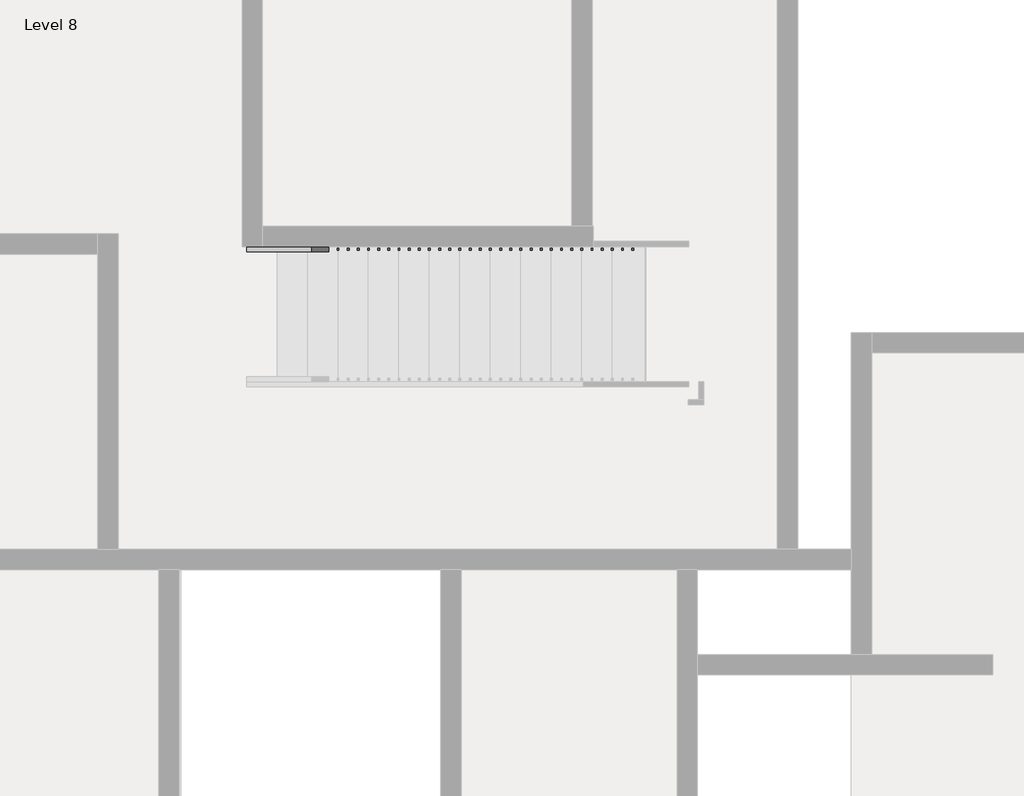
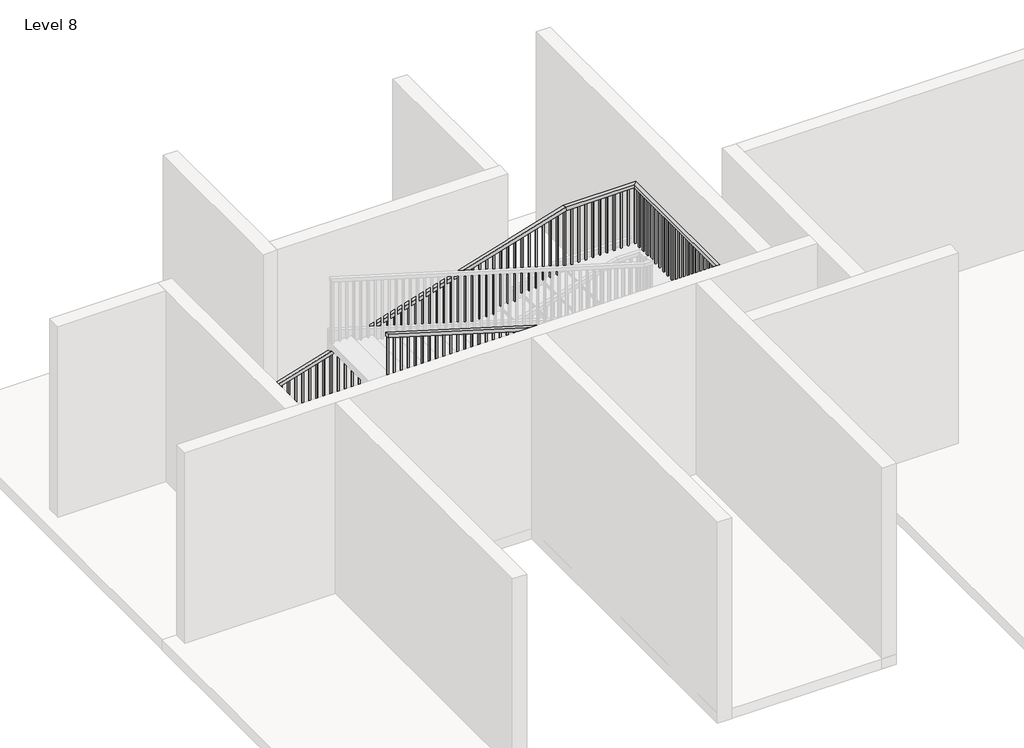
# One storey, part 10 of 14: 1 railing.
"""IFC4 building model written with IfcOpenShell, lengths in millimetres."""

from ifc_helpers import new_model, si_unit, frame, origin, place, context, project, spatial, polyline, outline, extrude, faceted_brep, element, save

model = new_model("IFC4")

# Units and contexts
model_context = context("Model", 3, world=origin())
ifc_project = project(units=[si_unit("LENGTHUNIT", "METRE", prefix="MILLI")], contexts=[model_context])

# Site, building, storey
site = spatial("IfcSite", under=ifc_project)
building = spatial("IfcBuilding", under=site)
storey = spatial("IfcBuildingStorey", under=building, Name="Level 8", Elevation=21336.0)

# Railing
placement = place(None, origin())
element("IfcRailing", 1, ObjectType="Handrail - Rectangular", at=placement, inside=storey, context=model_context, shape_type="SolidModel", body=[
    faceted_brep([(-5254.0891351, 12506.0715905, 22341.84), (-5254.0891351, 12506.0715905, 22288.8032429), (-5254.0891351, 12455.2715905, 22288.8032429), (-5254.0891351, 12455.2715905, 22341.84), (-986.8891351, 12506.0715905, 23622.0), (-979.4332782, 12506.0715905, 23571.2), (-979.4332782, 12455.2715905, 23571.2), (-986.8891351, 12455.2715905, 23622.0), (54.5108649, 12506.0715905, 23622.0), (54.5108649, 12506.0715905, 23571.2), (3.7108649, 12455.2715905, 23571.2), (3.7108649, 12455.2715905, 23622.0), (54.5108649, 9478.4949943, 23622.0), (54.5108649, 9478.4949943, 23571.2), (3.7108649, 9529.2949943, 23571.2), (3.7108649, 9529.2949943, 23622.0), (-682.0891351, 9478.4949943, 23622.0), (-689.544992, 9478.4949943, 23571.2), (-689.544992, 9529.2949943, 23571.2), (-682.0891351, 9529.2949943, 23622.0), (-5254.0891351, 9478.4949943, 24993.6), (-5254.0891351, 9529.2949943, 24993.6), (-5254.0891351, 9529.2949943, 24940.5632429), (-5254.0891351, 9478.4949943, 24940.5632429)], [[[0, 1, 2, 3]], [[1, 0, 4, 5]], [[2, 1, 5, 6]], [[3, 2, 6, 7]], [[0, 3, 7, 4]], [[5, 4, 8, 9]], [[6, 5, 9, 10]], [[7, 6, 10, 11]], [[4, 7, 11, 8]], [[9, 8, 12, 13]], [[10, 9, 13, 14]], [[11, 10, 14, 15]], [[8, 11, 15, 12]], [[13, 12, 16, 17]], [[14, 13, 17, 18]], [[15, 14, 18, 19]], [[12, 15, 19, 16]], [[20, 21, 22, 23]], [[17, 16, 20, 23]], [[18, 17, 23, 22]], [[19, 18, 22, 21]], [[16, 19, 21, 20]]]),
    extrude(outline(polyline([(24912.9407429, -5162.0141351), (23987.76, -5162.0141351), (23987.76, -5142.9641351), (24907.2257429, -5142.9641351), (24912.9407429, -5162.0141351)])), frame((0.0, 9494.3699943, 0.0), z_axis=(0.0, 1.0, 0.0), x_axis=(0.0, 0.0, 1.0)), (0.0, 0.0, 1.0), 19.05),
    extrude(outline(polyline([(24882.4607429, -5060.4141351), (23987.76, -5060.4141351), (23987.76, -5041.3641351), (24876.7457429, -5041.3641351), (24882.4607429, -5060.4141351)])), frame((0.0, 9494.3699943, 0.0), z_axis=(0.0, 1.0, 0.0), x_axis=(0.0, 0.0, 1.0)), (0.0, 0.0, 1.0), 19.05),
    extrude(outline(polyline([(24851.9807429, -4958.8141351), (23987.76, -4958.8141351), (23987.76, -4939.7641351), (24846.2657429, -4939.7641351), (24851.9807429, -4958.8141351)])), frame((0.0, 9494.3699943, 0.0), z_axis=(0.0, 1.0, 0.0), x_axis=(0.0, 0.0, 1.0)), (0.0, 0.0, 1.0), 19.05),
    extrude(outline(polyline([(24821.5007429, -4857.2141351), (23896.32, -4857.2141351), (23896.32, -4838.1641351), (24815.7857429, -4838.1641351), (24821.5007429, -4857.2141351)])), frame((0.0, 9494.3699943, 0.0), z_axis=(0.0, 1.0, 0.0), x_axis=(0.0, 0.0, 1.0)), (0.0, 0.0, 1.0), 19.05),
    extrude(outline(polyline([(24791.0207429, -4755.6141351), (23896.32, -4755.6141351), (23896.32, -4736.5641351), (24785.3057429, -4736.5641351), (24791.0207429, -4755.6141351)])), frame((0.0, 9494.3699943, 0.0), z_axis=(0.0, 1.0, 0.0), x_axis=(0.0, 0.0, 1.0)), (0.0, 0.0, 1.0), 19.05),
    extrude(outline(polyline([(24760.5407429, -4654.0141351), (23896.32, -4654.0141351), (23896.32, -4634.9641351), (24754.8257429, -4634.9641351), (24760.5407429, -4654.0141351)])), frame((0.0, 9494.3699943, 0.0), z_axis=(0.0, 1.0, 0.0), x_axis=(0.0, 0.0, 1.0)), (0.0, 0.0, 1.0), 19.05),
    extrude(outline(polyline([(24730.0607429, -4552.4141351), (23804.88, -4552.4141351), (23804.88, -4533.3641351), (24724.3457429, -4533.3641351), (24730.0607429, -4552.4141351)])), frame((0.0, 9494.3699943, 0.0), z_axis=(0.0, 1.0, 0.0), x_axis=(0.0, 0.0, 1.0)), (0.0, 0.0, 1.0), 19.05),
    extrude(outline(polyline([(24699.5807429, -4450.8141351), (23804.88, -4450.8141351), (23804.88, -4431.7641351), (24693.8657429, -4431.7641351), (24699.5807429, -4450.8141351)])), frame((0.0, 9494.3699943, 0.0), z_axis=(0.0, 1.0, 0.0), x_axis=(0.0, 0.0, 1.0)), (0.0, 0.0, 1.0), 19.05),
    extrude(outline(polyline([(24669.1007429, -4349.2141351), (23804.88, -4349.2141351), (23804.88, -4330.1641351), (24663.3857429, -4330.1641351), (24669.1007429, -4349.2141351)])), frame((0.0, 9494.3699943, 0.0), z_axis=(0.0, 1.0, 0.0), x_axis=(0.0, 0.0, 1.0)), (0.0, 0.0, 1.0), 19.05),
    extrude(outline(polyline([(24638.6207429, -4247.6141351), (23713.44, -4247.6141351), (23713.44, -4228.5641351), (24632.9057429, -4228.5641351), (24638.6207429, -4247.6141351)])), frame((0.0, 9494.3699943, 0.0), z_axis=(0.0, 1.0, 0.0), x_axis=(0.0, 0.0, 1.0)), (0.0, 0.0, 1.0), 19.05),
    extrude(outline(polyline([(24608.1407429, -4146.0141351), (23713.44, -4146.0141351), (23713.44, -4126.9641351), (24602.4257429, -4126.9641351), (24608.1407429, -4146.0141351)])), frame((0.0, 9494.3699943, 0.0), z_axis=(0.0, 1.0, 0.0), x_axis=(0.0, 0.0, 1.0)), (0.0, 0.0, 1.0), 19.05),
    extrude(outline(polyline([(24577.6607429, -4044.4141351), (23713.44, -4044.4141351), (23713.44, -4025.3641351), (24571.9457429, -4025.3641351), (24577.6607429, -4044.4141351)])), frame((0.0, 9494.3699943, 0.0), z_axis=(0.0, 1.0, 0.0), x_axis=(0.0, 0.0, 1.0)), (0.0, 0.0, 1.0), 19.05),
    extrude(outline(polyline([(24547.1807429, -3942.8141351), (23622.0, -3942.8141351), (23622.0, -3923.7641351), (24541.4657429, -3923.7641351), (24547.1807429, -3942.8141351)])), frame((0.0, 9494.3699943, 0.0), z_axis=(0.0, 1.0, 0.0), x_axis=(0.0, 0.0, 1.0)), (0.0, 0.0, 1.0), 19.05),
    extrude(outline(polyline([(24516.7007429, -3841.2141351), (23622.0, -3841.2141351), (23622.0, -3822.1641351), (24510.9857429, -3822.1641351), (24516.7007429, -3841.2141351)])), frame((0.0, 9494.3699943, 0.0), z_axis=(0.0, 1.0, 0.0), x_axis=(0.0, 0.0, 1.0)), (0.0, 0.0, 1.0), 19.05),
    extrude(outline(polyline([(24486.2207429, -3739.6141351), (23622.0, -3739.6141351), (23622.0, -3720.5641351), (24480.5057429, -3720.5641351), (24486.2207429, -3739.6141351)])), frame((0.0, 9494.3699943, 0.0), z_axis=(0.0, 1.0, 0.0), x_axis=(0.0, 0.0, 1.0)), (0.0, 0.0, 1.0), 19.05),
    extrude(outline(polyline([(24455.7407429, -3638.0141351), (23530.56, -3638.0141351), (23530.56, -3618.9641351), (24450.0257429, -3618.9641351), (24455.7407429, -3638.0141351)])), frame((0.0, 9494.3699943, 0.0), z_axis=(0.0, 1.0, 0.0), x_axis=(0.0, 0.0, 1.0)), (0.0, 0.0, 1.0), 19.05),
    extrude(outline(polyline([(24425.2607429, -3536.4141351), (23530.56, -3536.4141351), (23530.56, -3517.3641351), (24419.5457429, -3517.3641351), (24425.2607429, -3536.4141351)])), frame((0.0, 9494.3699943, 0.0), z_axis=(0.0, 1.0, 0.0), x_axis=(0.0, 0.0, 1.0)), (0.0, 0.0, 1.0), 19.05),
    extrude(outline(polyline([(24394.7807429, -3434.8141351), (23530.56, -3434.8141351), (23530.56, -3415.7641351), (24389.0657429, -3415.7641351), (24394.7807429, -3434.8141351)])), frame((0.0, 9494.3699943, 0.0), z_axis=(0.0, 1.0, 0.0), x_axis=(0.0, 0.0, 1.0)), (0.0, 0.0, 1.0), 19.05),
    extrude(outline(polyline([(24364.3007429, -3333.2141351), (23439.12, -3333.2141351), (23439.12, -3314.1641351), (24358.5857429, -3314.1641351), (24364.3007429, -3333.2141351)])), frame((0.0, 9494.3699943, 0.0), z_axis=(0.0, 1.0, 0.0), x_axis=(0.0, 0.0, 1.0)), (0.0, 0.0, 1.0), 19.05),
    extrude(outline(polyline([(24333.8207429, -3231.6141351), (23439.12, -3231.6141351), (23439.12, -3212.5641351), (24328.1057429, -3212.5641351), (24333.8207429, -3231.6141351)])), frame((0.0, 9494.3699943, 0.0), z_axis=(0.0, 1.0, 0.0), x_axis=(0.0, 0.0, 1.0)), (0.0, 0.0, 1.0), 19.05),
    extrude(outline(polyline([(24303.3407429, -3130.0141351), (23439.12, -3130.0141351), (23439.12, -3110.9641351), (24297.6257429, -3110.9641351), (24303.3407429, -3130.0141351)])), frame((0.0, 9494.3699943, 0.0), z_axis=(0.0, 1.0, 0.0), x_axis=(0.0, 0.0, 1.0)), (0.0, 0.0, 1.0), 19.05),
    extrude(outline(polyline([(24272.8607429, -3028.4141351), (23347.68, -3028.4141351), (23347.68, -3009.3641351), (24267.1457429, -3009.3641351), (24272.8607429, -3028.4141351)])), frame((0.0, 9494.3699943, 0.0), z_axis=(0.0, 1.0, 0.0), x_axis=(0.0, 0.0, 1.0)), (0.0, 0.0, 1.0), 19.05),
    extrude(outline(polyline([(24242.3807429, -2926.8141351), (23347.68, -2926.8141351), (23347.68, -2907.7641351), (24236.6657429, -2907.7641351), (24242.3807429, -2926.8141351)])), frame((0.0, 9494.3699943, 0.0), z_axis=(0.0, 1.0, 0.0), x_axis=(0.0, 0.0, 1.0)), (0.0, 0.0, 1.0), 19.05),
    extrude(outline(polyline([(24211.9007429, -2825.2141351), (23347.68, -2825.2141351), (23347.68, -2806.1641351), (24206.1857429, -2806.1641351), (24211.9007429, -2825.2141351)])), frame((0.0, 9494.3699943, 0.0), z_axis=(0.0, 1.0, 0.0), x_axis=(0.0, 0.0, 1.0)), (0.0, 0.0, 1.0), 19.05),
    extrude(outline(polyline([(24181.4207429, -2723.6141351), (23256.24, -2723.6141351), (23256.24, -2704.5641351), (24175.7057429, -2704.5641351), (24181.4207429, -2723.6141351)])), frame((0.0, 9494.3699943, 0.0), z_axis=(0.0, 1.0, 0.0), x_axis=(0.0, 0.0, 1.0)), (0.0, 0.0, 1.0), 19.05),
    extrude(outline(polyline([(24150.9407429, -2622.0141351), (23256.24, -2622.0141351), (23256.24, -2602.9641351), (24145.2257429, -2602.9641351), (24150.9407429, -2622.0141351)])), frame((0.0, 9494.3699943, 0.0), z_axis=(0.0, 1.0, 0.0), x_axis=(0.0, 0.0, 1.0)), (0.0, 0.0, 1.0), 19.05),
    extrude(outline(polyline([(24120.4607429, -2520.4141351), (23256.24, -2520.4141351), (23256.24, -2501.3641351), (24114.7457429, -2501.3641351), (24120.4607429, -2520.4141351)])), frame((0.0, 9494.3699943, 0.0), z_axis=(0.0, 1.0, 0.0), x_axis=(0.0, 0.0, 1.0)), (0.0, 0.0, 1.0), 19.05),
    extrude(outline(polyline([(24089.9807429, -2418.8141351), (23164.8, -2418.8141351), (23164.8, -2399.7641351), (24084.2657429, -2399.7641351), (24089.9807429, -2418.8141351)])), frame((0.0, 9494.3699943, 0.0), z_axis=(0.0, 1.0, 0.0), x_axis=(0.0, 0.0, 1.0)), (0.0, 0.0, 1.0), 19.05),
    extrude(outline(polyline([(24059.5007429, -2317.2141351), (23164.8, -2317.2141351), (23164.8, -2298.1641351), (24053.7857429, -2298.1641351), (24059.5007429, -2317.2141351)])), frame((0.0, 9494.3699943, 0.0), z_axis=(0.0, 1.0, 0.0), x_axis=(0.0, 0.0, 1.0)), (0.0, 0.0, 1.0), 19.05),
    extrude(outline(polyline([(24029.0207429, -2215.6141351), (23164.8, -2215.6141351), (23164.8, -2196.5641351), (24023.3057429, -2196.5641351), (24029.0207429, -2215.6141351)])), frame((0.0, 9494.3699943, 0.0), z_axis=(0.0, 1.0, 0.0), x_axis=(0.0, 0.0, 1.0)), (0.0, 0.0, 1.0), 19.05),
    extrude(outline(polyline([(23998.5407429, -2114.0141351), (23073.36, -2114.0141351), (23073.36, -2094.9641351), (23992.8257429, -2094.9641351), (23998.5407429, -2114.0141351)])), frame((0.0, 9494.3699943, 0.0), z_axis=(0.0, 1.0, 0.0), x_axis=(0.0, 0.0, 1.0)), (0.0, 0.0, 1.0), 19.05),
    extrude(outline(polyline([(23968.0607429, -2012.4141351), (23073.36, -2012.4141351), (23073.36, -1993.3641351), (23962.3457429, -1993.3641351), (23968.0607429, -2012.4141351)])), frame((0.0, 9494.3699943, 0.0), z_axis=(0.0, 1.0, 0.0), x_axis=(0.0, 0.0, 1.0)), (0.0, 0.0, 1.0), 19.05),
    extrude(outline(polyline([(23937.5807429, -1910.8141351), (23073.36, -1910.8141351), (23073.36, -1891.7641351), (23931.8657429, -1891.7641351), (23937.5807429, -1910.8141351)])), frame((0.0, 9494.3699943, 0.0), z_axis=(0.0, 1.0, 0.0), x_axis=(0.0, 0.0, 1.0)), (0.0, 0.0, 1.0), 19.05),
    extrude(outline(polyline([(23907.1007429, -1809.2141351), (22981.92, -1809.2141351), (22981.92, -1790.1641351), (23901.3857429, -1790.1641351), (23907.1007429, -1809.2141351)])), frame((0.0, 9494.3699943, 0.0), z_axis=(0.0, 1.0, 0.0), x_axis=(0.0, 0.0, 1.0)), (0.0, 0.0, 1.0), 19.05),
    extrude(outline(polyline([(23876.6207429, -1707.6141351), (22981.92, -1707.6141351), (22981.92, -1688.5641351), (23870.9057429, -1688.5641351), (23876.6207429, -1707.6141351)])), frame((0.0, 9494.3699943, 0.0), z_axis=(0.0, 1.0, 0.0), x_axis=(0.0, 0.0, 1.0)), (0.0, 0.0, 1.0), 19.05),
    extrude(outline(polyline([(23846.1407429, -1606.0141351), (22981.92, -1606.0141351), (22981.92, -1586.9641351), (23840.4257429, -1586.9641351), (23846.1407429, -1606.0141351)])), frame((0.0, 9494.3699943, 0.0), z_axis=(0.0, 1.0, 0.0), x_axis=(0.0, 0.0, 1.0)), (0.0, 0.0, 1.0), 19.05),
    extrude(outline(polyline([(23815.6607429, -1504.4141351), (22890.48, -1504.4141351), (22890.48, -1485.3641351), (23809.9457429, -1485.3641351), (23815.6607429, -1504.4141351)])), frame((0.0, 9494.3699943, 0.0), z_axis=(0.0, 1.0, 0.0), x_axis=(0.0, 0.0, 1.0)), (0.0, 0.0, 1.0), 19.05),
    extrude(outline(polyline([(23785.1807429, -1402.8141351), (22890.48, -1402.8141351), (22890.48, -1383.7641351), (23779.4657429, -1383.7641351), (23785.1807429, -1402.8141351)])), frame((0.0, 9494.3699943, 0.0), z_axis=(0.0, 1.0, 0.0), x_axis=(0.0, 0.0, 1.0)), (0.0, 0.0, 1.0), 19.05),
    extrude(outline(polyline([(23754.7007429, -1301.2141351), (22890.48, -1301.2141351), (22890.48, -1282.1641351), (23748.9857429, -1282.1641351), (23754.7007429, -1301.2141351)])), frame((0.0, 9494.3699943, 0.0), z_axis=(0.0, 1.0, 0.0), x_axis=(0.0, 0.0, 1.0)), (0.0, 0.0, 1.0), 19.05),
    extrude(outline(polyline([(23724.2207429, -1199.6141351), (22799.04, -1199.6141351), (22799.04, -1180.5641351), (23718.5057429, -1180.5641351), (23724.2207429, -1199.6141351)])), frame((0.0, 9494.3699943, 0.0), z_axis=(0.0, 1.0, 0.0), x_axis=(0.0, 0.0, 1.0)), (0.0, 0.0, 1.0), 19.05),
    extrude(outline(polyline([(23693.7407429, -1098.0141351), (22799.04, -1098.0141351), (22799.04, -1078.9641351), (23688.0257429, -1078.9641351), (23693.7407429, -1098.0141351)])), frame((0.0, 9494.3699943, 0.0), z_axis=(0.0, 1.0, 0.0), x_axis=(0.0, 0.0, 1.0)), (0.0, 0.0, 1.0), 19.05),
    extrude(outline(polyline([(23663.2607429, -996.4141351), (22799.04, -996.4141351), (22799.04, -977.3641351), (23657.5457429, -977.3641351), (23663.2607429, -996.4141351)])), frame((0.0, 9494.3699943, 0.0), z_axis=(0.0, 1.0, 0.0), x_axis=(0.0, 0.0, 1.0)), (0.0, 0.0, 1.0), 19.05),
    extrude(outline(polyline([(23632.7807429, -894.8141351), (22707.6, -894.8141351), (22707.6, -875.7641351), (23627.0657429, -875.7641351), (23632.7807429, -894.8141351)])), frame((0.0, 9494.3699943, 0.0), z_axis=(0.0, 1.0, 0.0), x_axis=(0.0, 0.0, 1.0)), (0.0, 0.0, 1.0), 19.05),
    extrude(outline(polyline([(23602.3007429, -793.2141351), (22707.6, -793.2141351), (22707.6, -774.1641351), (23596.5857429, -774.1641351), (23602.3007429, -793.2141351)])), frame((0.0, 9494.3699943, 0.0), z_axis=(0.0, 1.0, 0.0), x_axis=(0.0, 0.0, 1.0)), (0.0, 0.0, 1.0), 19.05),
    extrude(outline(polyline([(-672.5641351, 9494.3699943), (-691.6141351, 9494.3699943), (-691.6141351, 9513.4199943), (-672.5641351, 9513.4199943), (-672.5641351, 9494.3699943)])), frame((0.0, 0.0, 22707.6), z_axis=(0.0, 0.0, 1.0), x_axis=(1.0, 0.0, 0.0)), (0.0, 0.0, 1.0), 863.6),
    extrude(outline(polyline([(-570.9641351, 9494.3699943), (-590.0141351, 9494.3699943), (-590.0141351, 9513.4199943), (-570.9641351, 9513.4199943), (-570.9641351, 9494.3699943)])), frame((0.0, 0.0, 22707.6), z_axis=(0.0, 0.0, 1.0), x_axis=(1.0, 0.0, 0.0)), (0.0, 0.0, 1.0), 863.6),
    extrude(outline(polyline([(-469.3641351, 9494.3699943), (-488.4141351, 9494.3699943), (-488.4141351, 9513.4199943), (-469.3641351, 9513.4199943), (-469.3641351, 9494.3699943)])), frame((0.0, 0.0, 22707.6), z_axis=(0.0, 0.0, 1.0), x_axis=(1.0, 0.0, 0.0)), (0.0, 0.0, 1.0), 863.6),
    extrude(outline(polyline([(-367.7641351, 9494.3699943), (-386.8141351, 9494.3699943), (-386.8141351, 9513.4199943), (-367.7641351, 9513.4199943), (-367.7641351, 9494.3699943)])), frame((0.0, 0.0, 22707.6), z_axis=(0.0, 0.0, 1.0), x_axis=(1.0, 0.0, 0.0)), (0.0, 0.0, 1.0), 863.6),
    extrude(outline(polyline([(-266.1641351, 9494.3699943), (-285.2141351, 9494.3699943), (-285.2141351, 9513.4199943), (-266.1641351, 9513.4199943), (-266.1641351, 9494.3699943)])), frame((0.0, 0.0, 22707.6), z_axis=(0.0, 0.0, 1.0), x_axis=(1.0, 0.0, 0.0)), (0.0, 0.0, 1.0), 863.6),
    extrude(outline(polyline([(-164.5641351, 9494.3699943), (-183.6141351, 9494.3699943), (-183.6141351, 9513.4199943), (-164.5641351, 9513.4199943), (-164.5641351, 9494.3699943)])), frame((0.0, 0.0, 22707.6), z_axis=(0.0, 0.0, 1.0), x_axis=(1.0, 0.0, 0.0)), (0.0, 0.0, 1.0), 863.6),
    extrude(outline(polyline([(-62.9641351, 9494.3699943), (-82.0141351, 9494.3699943), (-82.0141351, 9513.4199943), (-62.9641351, 9513.4199943), (-62.9641351, 9494.3699943)])), frame((0.0, 0.0, 22707.6), z_axis=(0.0, 0.0, 1.0), x_axis=(1.0, 0.0, 0.0)), (0.0, 0.0, 1.0), 863.6),
    extrude(outline(polyline([(38.6358649, 9543.7965905), (38.6358649, 9524.7465905), (19.5858649, 9524.7465905), (19.5858649, 9543.7965905), (38.6358649, 9543.7965905)])), frame((0.0, 0.0, 22707.6), z_axis=(0.0, 0.0, 1.0), x_axis=(1.0, 0.0, 0.0)), (0.0, 0.0, 1.0), 863.6),
    extrude(outline(polyline([(38.6358649, 9645.3965905), (38.6358649, 9626.3465905), (19.5858649, 9626.3465905), (19.5858649, 9645.3965905), (38.6358649, 9645.3965905)])), frame((0.0, 0.0, 22707.6), z_axis=(0.0, 0.0, 1.0), x_axis=(1.0, 0.0, 0.0)), (0.0, 0.0, 1.0), 863.6),
    extrude(outline(polyline([(38.6358649, 9746.9965905), (38.6358649, 9727.9465905), (19.5858649, 9727.9465905), (19.5858649, 9746.9965905), (38.6358649, 9746.9965905)])), frame((0.0, 0.0, 22707.6), z_axis=(0.0, 0.0, 1.0), x_axis=(1.0, 0.0, 0.0)), (0.0, 0.0, 1.0), 863.6),
    extrude(outline(polyline([(38.6358649, 9848.5965905), (38.6358649, 9829.5465905), (19.5858649, 9829.5465905), (19.5858649, 9848.5965905), (38.6358649, 9848.5965905)])), frame((0.0, 0.0, 22707.6), z_axis=(0.0, 0.0, 1.0), x_axis=(1.0, 0.0, 0.0)), (0.0, 0.0, 1.0), 863.6),
    extrude(outline(polyline([(38.6358649, 9950.1965905), (38.6358649, 9931.1465905), (19.5858649, 9931.1465905), (19.5858649, 9950.1965905), (38.6358649, 9950.1965905)])), frame((0.0, 0.0, 22707.6), z_axis=(0.0, 0.0, 1.0), x_axis=(1.0, 0.0, 0.0)), (0.0, 0.0, 1.0), 863.6),
    extrude(outline(polyline([(38.6358649, 10051.7965905), (38.6358649, 10032.7465905), (19.5858649, 10032.7465905), (19.5858649, 10051.7965905), (38.6358649, 10051.7965905)])), frame((0.0, 0.0, 22707.6), z_axis=(0.0, 0.0, 1.0), x_axis=(1.0, 0.0, 0.0)), (0.0, 0.0, 1.0), 863.6),
    extrude(outline(polyline([(38.6358649, 10153.3965905), (38.6358649, 10134.3465905), (19.5858649, 10134.3465905), (19.5858649, 10153.3965905), (38.6358649, 10153.3965905)])), frame((0.0, 0.0, 22707.6), z_axis=(0.0, 0.0, 1.0), x_axis=(1.0, 0.0, 0.0)), (0.0, 0.0, 1.0), 863.6),
    extrude(outline(polyline([(38.6358649, 10254.9965905), (38.6358649, 10235.9465905), (19.5858649, 10235.9465905), (19.5858649, 10254.9965905), (38.6358649, 10254.9965905)])), frame((0.0, 0.0, 22707.6), z_axis=(0.0, 0.0, 1.0), x_axis=(1.0, 0.0, 0.0)), (0.0, 0.0, 1.0), 863.6),
    extrude(outline(polyline([(38.6358649, 10356.5965905), (38.6358649, 10337.5465905), (19.5858649, 10337.5465905), (19.5858649, 10356.5965905), (38.6358649, 10356.5965905)])), frame((0.0, 0.0, 22707.6), z_axis=(0.0, 0.0, 1.0), x_axis=(1.0, 0.0, 0.0)), (0.0, 0.0, 1.0), 863.6),
    extrude(outline(polyline([(38.6358649, 10458.1965905), (38.6358649, 10439.1465905), (19.5858649, 10439.1465905), (19.5858649, 10458.1965905), (38.6358649, 10458.1965905)])), frame((0.0, 0.0, 22707.6), z_axis=(0.0, 0.0, 1.0), x_axis=(1.0, 0.0, 0.0)), (0.0, 0.0, 1.0), 863.6),
    extrude(outline(polyline([(38.6358649, 10559.7965905), (38.6358649, 10540.7465905), (19.5858649, 10540.7465905), (19.5858649, 10559.7965905), (38.6358649, 10559.7965905)])), frame((0.0, 0.0, 22707.6), z_axis=(0.0, 0.0, 1.0), x_axis=(1.0, 0.0, 0.0)), (0.0, 0.0, 1.0), 863.6),
    extrude(outline(polyline([(38.6358649, 10661.3965905), (38.6358649, 10642.3465905), (19.5858649, 10642.3465905), (19.5858649, 10661.3965905), (38.6358649, 10661.3965905)])), frame((0.0, 0.0, 22707.6), z_axis=(0.0, 0.0, 1.0), x_axis=(1.0, 0.0, 0.0)), (0.0, 0.0, 1.0), 863.6),
    extrude(outline(polyline([(38.6358649, 10762.9965905), (38.6358649, 10743.9465905), (19.5858649, 10743.9465905), (19.5858649, 10762.9965905), (38.6358649, 10762.9965905)])), frame((0.0, 0.0, 22707.6), z_axis=(0.0, 0.0, 1.0), x_axis=(1.0, 0.0, 0.0)), (0.0, 0.0, 1.0), 863.6),
    extrude(outline(polyline([(38.6358649, 10864.5965905), (38.6358649, 10845.5465905), (19.5858649, 10845.5465905), (19.5858649, 10864.5965905), (38.6358649, 10864.5965905)])), frame((0.0, 0.0, 22707.6), z_axis=(0.0, 0.0, 1.0), x_axis=(1.0, 0.0, 0.0)), (0.0, 0.0, 1.0), 863.6),
    extrude(outline(polyline([(38.6358649, 10966.1965905), (38.6358649, 10947.1465905), (19.5858649, 10947.1465905), (19.5858649, 10966.1965905), (38.6358649, 10966.1965905)])), frame((0.0, 0.0, 22707.6), z_axis=(0.0, 0.0, 1.0), x_axis=(1.0, 0.0, 0.0)), (0.0, 0.0, 1.0), 863.6),
    extrude(outline(polyline([(38.6358649, 11067.7965905), (38.6358649, 11048.7465905), (19.5858649, 11048.7465905), (19.5858649, 11067.7965905), (38.6358649, 11067.7965905)])), frame((0.0, 0.0, 22707.6), z_axis=(0.0, 0.0, 1.0), x_axis=(1.0, 0.0, 0.0)), (0.0, 0.0, 1.0), 863.6),
    extrude(outline(polyline([(38.6358649, 11169.3965905), (38.6358649, 11150.3465905), (19.5858649, 11150.3465905), (19.5858649, 11169.3965905), (38.6358649, 11169.3965905)])), frame((0.0, 0.0, 22707.6), z_axis=(0.0, 0.0, 1.0), x_axis=(1.0, 0.0, 0.0)), (0.0, 0.0, 1.0), 863.6),
    extrude(outline(polyline([(38.6358649, 11270.9965905), (38.6358649, 11251.9465905), (19.5858649, 11251.9465905), (19.5858649, 11270.9965905), (38.6358649, 11270.9965905)])), frame((0.0, 0.0, 22707.6), z_axis=(0.0, 0.0, 1.0), x_axis=(1.0, 0.0, 0.0)), (0.0, 0.0, 1.0), 863.6),
    extrude(outline(polyline([(38.6358649, 11372.5965905), (38.6358649, 11353.5465905), (19.5858649, 11353.5465905), (19.5858649, 11372.5965905), (38.6358649, 11372.5965905)])), frame((0.0, 0.0, 22707.6), z_axis=(0.0, 0.0, 1.0), x_axis=(1.0, 0.0, 0.0)), (0.0, 0.0, 1.0), 863.6),
    extrude(outline(polyline([(38.6358649, 11474.1965905), (38.6358649, 11455.1465905), (19.5858649, 11455.1465905), (19.5858649, 11474.1965905), (38.6358649, 11474.1965905)])), frame((0.0, 0.0, 22707.6), z_axis=(0.0, 0.0, 1.0), x_axis=(1.0, 0.0, 0.0)), (0.0, 0.0, 1.0), 863.6),
    extrude(outline(polyline([(38.6358649, 11575.7965905), (38.6358649, 11556.7465905), (19.5858649, 11556.7465905), (19.5858649, 11575.7965905), (38.6358649, 11575.7965905)])), frame((0.0, 0.0, 22707.6), z_axis=(0.0, 0.0, 1.0), x_axis=(1.0, 0.0, 0.0)), (0.0, 0.0, 1.0), 863.6),
    extrude(outline(polyline([(38.6358649, 11677.3965905), (38.6358649, 11658.3465905), (19.5858649, 11658.3465905), (19.5858649, 11677.3965905), (38.6358649, 11677.3965905)])), frame((0.0, 0.0, 22707.6), z_axis=(0.0, 0.0, 1.0), x_axis=(1.0, 0.0, 0.0)), (0.0, 0.0, 1.0), 863.6),
    extrude(outline(polyline([(38.6358649, 11778.9965905), (38.6358649, 11759.9465905), (19.5858649, 11759.9465905), (19.5858649, 11778.9965905), (38.6358649, 11778.9965905)])), frame((0.0, 0.0, 22707.6), z_axis=(0.0, 0.0, 1.0), x_axis=(1.0, 0.0, 0.0)), (0.0, 0.0, 1.0), 863.6),
    extrude(outline(polyline([(38.6358649, 11880.5965905), (38.6358649, 11861.5465905), (19.5858649, 11861.5465905), (19.5858649, 11880.5965905), (38.6358649, 11880.5965905)])), frame((0.0, 0.0, 22707.6), z_axis=(0.0, 0.0, 1.0), x_axis=(1.0, 0.0, 0.0)), (0.0, 0.0, 1.0), 863.6),
    extrude(outline(polyline([(38.6358649, 11982.1965905), (38.6358649, 11963.1465905), (19.5858649, 11963.1465905), (19.5858649, 11982.1965905), (38.6358649, 11982.1965905)])), frame((0.0, 0.0, 22707.6), z_axis=(0.0, 0.0, 1.0), x_axis=(1.0, 0.0, 0.0)), (0.0, 0.0, 1.0), 863.6),
    extrude(outline(polyline([(38.6358649, 12083.7965905), (38.6358649, 12064.7465905), (19.5858649, 12064.7465905), (19.5858649, 12083.7965905), (38.6358649, 12083.7965905)])), frame((0.0, 0.0, 22707.6), z_axis=(0.0, 0.0, 1.0), x_axis=(1.0, 0.0, 0.0)), (0.0, 0.0, 1.0), 863.6),
    extrude(outline(polyline([(38.6358649, 12185.3965905), (38.6358649, 12166.3465905), (19.5858649, 12166.3465905), (19.5858649, 12185.3965905), (38.6358649, 12185.3965905)])), frame((0.0, 0.0, 22707.6), z_axis=(0.0, 0.0, 1.0), x_axis=(1.0, 0.0, 0.0)), (0.0, 0.0, 1.0), 863.6),
    extrude(outline(polyline([(38.6358649, 12286.9965905), (38.6358649, 12267.9465905), (19.5858649, 12267.9465905), (19.5858649, 12286.9965905), (38.6358649, 12286.9965905)])), frame((0.0, 0.0, 22707.6), z_axis=(0.0, 0.0, 1.0), x_axis=(1.0, 0.0, 0.0)), (0.0, 0.0, 1.0), 863.6),
    extrude(outline(polyline([(38.6358649, 12388.5965905), (38.6358649, 12369.5465905), (19.5858649, 12369.5465905), (19.5858649, 12388.5965905), (38.6358649, 12388.5965905)])), frame((0.0, 0.0, 22707.6), z_axis=(0.0, 0.0, 1.0), x_axis=(1.0, 0.0, 0.0)), (0.0, 0.0, 1.0), 863.6),
    extrude(outline(polyline([(-82.0141351, 12490.1965905), (-62.9641351, 12490.1965905), (-62.9641351, 12471.1465905), (-82.0141351, 12471.1465905), (-82.0141351, 12490.1965905)])), frame((0.0, 0.0, 22707.6), z_axis=(0.0, 0.0, 1.0), x_axis=(1.0, 0.0, 0.0)), (0.0, 0.0, 1.0), 863.6),
    extrude(outline(polyline([(-183.6141351, 12490.1965905), (-164.5641351, 12490.1965905), (-164.5641351, 12471.1465905), (-183.6141351, 12471.1465905), (-183.6141351, 12490.1965905)])), frame((0.0, 0.0, 22707.6), z_axis=(0.0, 0.0, 1.0), x_axis=(1.0, 0.0, 0.0)), (0.0, 0.0, 1.0), 863.6),
    extrude(outline(polyline([(-285.2141351, 12490.1965905), (-266.1641351, 12490.1965905), (-266.1641351, 12471.1465905), (-285.2141351, 12471.1465905), (-285.2141351, 12490.1965905)])), frame((0.0, 0.0, 22707.6), z_axis=(0.0, 0.0, 1.0), x_axis=(1.0, 0.0, 0.0)), (0.0, 0.0, 1.0), 863.6),
    extrude(outline(polyline([(-386.8141351, 12490.1965905), (-367.7641351, 12490.1965905), (-367.7641351, 12471.1465905), (-386.8141351, 12471.1465905), (-386.8141351, 12490.1965905)])), frame((0.0, 0.0, 22707.6), z_axis=(0.0, 0.0, 1.0), x_axis=(1.0, 0.0, 0.0)), (0.0, 0.0, 1.0), 863.6),
    extrude(outline(polyline([(-488.4141351, 12490.1965905), (-469.3641351, 12490.1965905), (-469.3641351, 12471.1465905), (-488.4141351, 12471.1465905), (-488.4141351, 12490.1965905)])), frame((0.0, 0.0, 22707.6), z_axis=(0.0, 0.0, 1.0), x_axis=(1.0, 0.0, 0.0)), (0.0, 0.0, 1.0), 863.6),
    extrude(outline(polyline([(-590.0141351, 12490.1965905), (-570.9641351, 12490.1965905), (-570.9641351, 12471.1465905), (-590.0141351, 12471.1465905), (-590.0141351, 12490.1965905)])), frame((0.0, 0.0, 22707.6), z_axis=(0.0, 0.0, 1.0), x_axis=(1.0, 0.0, 0.0)), (0.0, 0.0, 1.0), 863.6),
    extrude(outline(polyline([(-691.6141351, 12490.1965905), (-672.5641351, 12490.1965905), (-672.5641351, 12471.1465905), (-691.6141351, 12471.1465905), (-691.6141351, 12490.1965905)])), frame((0.0, 0.0, 22707.6), z_axis=(0.0, 0.0, 1.0), x_axis=(1.0, 0.0, 0.0)), (0.0, 0.0, 1.0), 863.6),
    extrude(outline(polyline([(-793.2141351, 12490.1965905), (-774.1641351, 12490.1965905), (-774.1641351, 12471.1465905), (-793.2141351, 12471.1465905), (-793.2141351, 12490.1965905)])), frame((0.0, 0.0, 22707.6), z_axis=(0.0, 0.0, 1.0), x_axis=(1.0, 0.0, 0.0)), (0.0, 0.0, 1.0), 863.6),
    extrude(outline(polyline([(-894.8141351, 12490.1965905), (-875.7641351, 12490.1965905), (-875.7641351, 12471.1465905), (-894.8141351, 12471.1465905), (-894.8141351, 12490.1965905)])), frame((0.0, 0.0, 22707.6), z_axis=(0.0, 0.0, 1.0), x_axis=(1.0, 0.0, 0.0)), (0.0, 0.0, 1.0), 863.6),
    extrude(outline(polyline([(23566.1057429, -996.4141351), (22707.6, -996.4141351), (22707.6, -977.3641351), (23571.8207429, -977.3641351), (23566.1057429, -996.4141351)])), frame((0.0, 12471.1465905, 0.0), z_axis=(0.0, 1.0, 0.0), x_axis=(0.0, 0.0, 1.0)), (0.0, 0.0, 1.0), 19.05),
    extrude(outline(polyline([(23535.6257429, -1098.0141351), (22616.16, -1098.0141351), (22616.16, -1078.9641351), (23541.3407429, -1078.9641351), (23535.6257429, -1098.0141351)])), frame((0.0, 12471.1465905, 0.0), z_axis=(0.0, 1.0, 0.0), x_axis=(0.0, 0.0, 1.0)), (0.0, 0.0, 1.0), 19.05),
    extrude(outline(polyline([(23505.1457429, -1199.6141351), (22616.16, -1199.6141351), (22616.16, -1180.5641351), (23510.8607429, -1180.5641351), (23505.1457429, -1199.6141351)])), frame((0.0, 12471.1465905, 0.0), z_axis=(0.0, 1.0, 0.0), x_axis=(0.0, 0.0, 1.0)), (0.0, 0.0, 1.0), 19.05),
    extrude(outline(polyline([(23474.6657429, -1301.2141351), (22616.16, -1301.2141351), (22616.16, -1282.1641351), (23480.3807429, -1282.1641351), (23474.6657429, -1301.2141351)])), frame((0.0, 12471.1465905, 0.0), z_axis=(0.0, 1.0, 0.0), x_axis=(0.0, 0.0, 1.0)), (0.0, 0.0, 1.0), 19.05),
    extrude(outline(polyline([(23444.1857429, -1402.8141351), (22524.72, -1402.8141351), (22524.72, -1383.7641351), (23449.9007429, -1383.7641351), (23444.1857429, -1402.8141351)])), frame((0.0, 12471.1465905, 0.0), z_axis=(0.0, 1.0, 0.0), x_axis=(0.0, 0.0, 1.0)), (0.0, 0.0, 1.0), 19.05),
    extrude(outline(polyline([(23413.7057429, -1504.4141351), (22524.72, -1504.4141351), (22524.72, -1485.3641351), (23419.4207429, -1485.3641351), (23413.7057429, -1504.4141351)])), frame((0.0, 12471.1465905, 0.0), z_axis=(0.0, 1.0, 0.0), x_axis=(0.0, 0.0, 1.0)), (0.0, 0.0, 1.0), 19.05),
    extrude(outline(polyline([(23383.2257429, -1606.0141351), (22524.72, -1606.0141351), (22524.72, -1586.9641351), (23388.9407429, -1586.9641351), (23383.2257429, -1606.0141351)])), frame((0.0, 12471.1465905, 0.0), z_axis=(0.0, 1.0, 0.0), x_axis=(0.0, 0.0, 1.0)), (0.0, 0.0, 1.0), 19.05),
    extrude(outline(polyline([(23352.7457429, -1707.6141351), (22433.28, -1707.6141351), (22433.28, -1688.5641351), (23358.4607429, -1688.5641351), (23352.7457429, -1707.6141351)])), frame((0.0, 12471.1465905, 0.0), z_axis=(0.0, 1.0, 0.0), x_axis=(0.0, 0.0, 1.0)), (0.0, 0.0, 1.0), 19.05),
    extrude(outline(polyline([(23322.2657429, -1809.2141351), (22433.28, -1809.2141351), (22433.28, -1790.1641351), (23327.9807429, -1790.1641351), (23322.2657429, -1809.2141351)])), frame((0.0, 12471.1465905, 0.0), z_axis=(0.0, 1.0, 0.0), x_axis=(0.0, 0.0, 1.0)), (0.0, 0.0, 1.0), 19.05),
    extrude(outline(polyline([(23291.7857429, -1910.8141351), (22433.28, -1910.8141351), (22433.28, -1891.7641351), (23297.5007429, -1891.7641351), (23291.7857429, -1910.8141351)])), frame((0.0, 12471.1465905, 0.0), z_axis=(0.0, 1.0, 0.0), x_axis=(0.0, 0.0, 1.0)), (0.0, 0.0, 1.0), 19.05),
    extrude(outline(polyline([(23261.3057429, -2012.4141351), (22341.84, -2012.4141351), (22341.84, -1993.3641351), (23267.0207429, -1993.3641351), (23261.3057429, -2012.4141351)])), frame((0.0, 12471.1465905, 0.0), z_axis=(0.0, 1.0, 0.0), x_axis=(0.0, 0.0, 1.0)), (0.0, 0.0, 1.0), 19.05),
    extrude(outline(polyline([(23230.8257429, -2114.0141351), (22341.84, -2114.0141351), (22341.84, -2094.9641351), (23236.5407429, -2094.9641351), (23230.8257429, -2114.0141351)])), frame((0.0, 12471.1465905, 0.0), z_axis=(0.0, 1.0, 0.0), x_axis=(0.0, 0.0, 1.0)), (0.0, 0.0, 1.0), 19.05),
    extrude(outline(polyline([(23200.3457429, -2215.6141351), (22341.84, -2215.6141351), (22341.84, -2196.5641351), (23206.0607429, -2196.5641351), (23200.3457429, -2215.6141351)])), frame((0.0, 12471.1465905, 0.0), z_axis=(0.0, 1.0, 0.0), x_axis=(0.0, 0.0, 1.0)), (0.0, 0.0, 1.0), 19.05),
    extrude(outline(polyline([(23169.8657429, -2317.2141351), (22250.4, -2317.2141351), (22250.4, -2298.1641351), (23175.5807429, -2298.1641351), (23169.8657429, -2317.2141351)])), frame((0.0, 12471.1465905, 0.0), z_axis=(0.0, 1.0, 0.0), x_axis=(0.0, 0.0, 1.0)), (0.0, 0.0, 1.0), 19.05),
    extrude(outline(polyline([(23139.3857429, -2418.8141351), (22250.4, -2418.8141351), (22250.4, -2399.7641351), (23145.1007429, -2399.7641351), (23139.3857429, -2418.8141351)])), frame((0.0, 12471.1465905, 0.0), z_axis=(0.0, 1.0, 0.0), x_axis=(0.0, 0.0, 1.0)), (0.0, 0.0, 1.0), 19.05),
    extrude(outline(polyline([(23108.9057429, -2520.4141351), (22250.4, -2520.4141351), (22250.4, -2501.3641351), (23114.6207429, -2501.3641351), (23108.9057429, -2520.4141351)])), frame((0.0, 12471.1465905, 0.0), z_axis=(0.0, 1.0, 0.0), x_axis=(0.0, 0.0, 1.0)), (0.0, 0.0, 1.0), 19.05),
    extrude(outline(polyline([(23078.4257429, -2622.0141351), (22158.96, -2622.0141351), (22158.96, -2602.9641351), (23084.1407429, -2602.9641351), (23078.4257429, -2622.0141351)])), frame((0.0, 12471.1465905, 0.0), z_axis=(0.0, 1.0, 0.0), x_axis=(0.0, 0.0, 1.0)), (0.0, 0.0, 1.0), 19.05),
    extrude(outline(polyline([(23047.9457429, -2723.6141351), (22158.96, -2723.6141351), (22158.96, -2704.5641351), (23053.6607429, -2704.5641351), (23047.9457429, -2723.6141351)])), frame((0.0, 12471.1465905, 0.0), z_axis=(0.0, 1.0, 0.0), x_axis=(0.0, 0.0, 1.0)), (0.0, 0.0, 1.0), 19.05),
    extrude(outline(polyline([(23017.4657429, -2825.2141351), (22158.96, -2825.2141351), (22158.96, -2806.1641351), (23023.1807429, -2806.1641351), (23017.4657429, -2825.2141351)])), frame((0.0, 12471.1465905, 0.0), z_axis=(0.0, 1.0, 0.0), x_axis=(0.0, 0.0, 1.0)), (0.0, 0.0, 1.0), 19.05),
    extrude(outline(polyline([(22986.9857429, -2926.8141351), (22067.52, -2926.8141351), (22067.52, -2907.7641351), (22992.7007429, -2907.7641351), (22986.9857429, -2926.8141351)])), frame((0.0, 12471.1465905, 0.0), z_axis=(0.0, 1.0, 0.0), x_axis=(0.0, 0.0, 1.0)), (0.0, 0.0, 1.0), 19.05),
    extrude(outline(polyline([(22956.5057429, -3028.4141351), (22067.52, -3028.4141351), (22067.52, -3009.3641351), (22962.2207429, -3009.3641351), (22956.5057429, -3028.4141351)])), frame((0.0, 12471.1465905, 0.0), z_axis=(0.0, 1.0, 0.0), x_axis=(0.0, 0.0, 1.0)), (0.0, 0.0, 1.0), 19.05),
    extrude(outline(polyline([(22926.0257429, -3130.0141351), (22067.52, -3130.0141351), (22067.52, -3110.9641351), (22931.7407429, -3110.9641351), (22926.0257429, -3130.0141351)])), frame((0.0, 12471.1465905, 0.0), z_axis=(0.0, 1.0, 0.0), x_axis=(0.0, 0.0, 1.0)), (0.0, 0.0, 1.0), 19.05),
    extrude(outline(polyline([(22895.5457429, -3231.6141351), (21976.08, -3231.6141351), (21976.08, -3212.5641351), (22901.2607429, -3212.5641351), (22895.5457429, -3231.6141351)])), frame((0.0, 12471.1465905, 0.0), z_axis=(0.0, 1.0, 0.0), x_axis=(0.0, 0.0, 1.0)), (0.0, 0.0, 1.0), 19.05),
    extrude(outline(polyline([(22865.0657429, -3333.2141351), (21976.08, -3333.2141351), (21976.08, -3314.1641351), (22870.7807429, -3314.1641351), (22865.0657429, -3333.2141351)])), frame((0.0, 12471.1465905, 0.0), z_axis=(0.0, 1.0, 0.0), x_axis=(0.0, 0.0, 1.0)), (0.0, 0.0, 1.0), 19.05),
    extrude(outline(polyline([(22834.5857429, -3434.8141351), (21976.08, -3434.8141351), (21976.08, -3415.7641351), (22840.3007429, -3415.7641351), (22834.5857429, -3434.8141351)])), frame((0.0, 12471.1465905, 0.0), z_axis=(0.0, 1.0, 0.0), x_axis=(0.0, 0.0, 1.0)), (0.0, 0.0, 1.0), 19.05),
    extrude(outline(polyline([(22804.1057429, -3536.4141351), (21884.64, -3536.4141351), (21884.64, -3517.3641351), (22809.8207429, -3517.3641351), (22804.1057429, -3536.4141351)])), frame((0.0, 12471.1465905, 0.0), z_axis=(0.0, 1.0, 0.0), x_axis=(0.0, 0.0, 1.0)), (0.0, 0.0, 1.0), 19.05),
    extrude(outline(polyline([(22773.6257429, -3638.0141351), (21884.64, -3638.0141351), (21884.64, -3618.9641351), (22779.3407429, -3618.9641351), (22773.6257429, -3638.0141351)])), frame((0.0, 12471.1465905, 0.0), z_axis=(0.0, 1.0, 0.0), x_axis=(0.0, 0.0, 1.0)), (0.0, 0.0, 1.0), 19.05),
    extrude(outline(polyline([(22743.1457429, -3739.6141351), (21884.64, -3739.6141351), (21884.64, -3720.5641351), (22748.8607429, -3720.5641351), (22743.1457429, -3739.6141351)])), frame((0.0, 12471.1465905, 0.0), z_axis=(0.0, 1.0, 0.0), x_axis=(0.0, 0.0, 1.0)), (0.0, 0.0, 1.0), 19.05),
    extrude(outline(polyline([(22712.6657429, -3841.2141351), (21793.2, -3841.2141351), (21793.2, -3822.1641351), (22718.3807429, -3822.1641351), (22712.6657429, -3841.2141351)])), frame((0.0, 12471.1465905, 0.0), z_axis=(0.0, 1.0, 0.0), x_axis=(0.0, 0.0, 1.0)), (0.0, 0.0, 1.0), 19.05),
    extrude(outline(polyline([(22682.1857429, -3942.8141351), (21793.2, -3942.8141351), (21793.2, -3923.7641351), (22687.9007429, -3923.7641351), (22682.1857429, -3942.8141351)])), frame((0.0, 12471.1465905, 0.0), z_axis=(0.0, 1.0, 0.0), x_axis=(0.0, 0.0, 1.0)), (0.0, 0.0, 1.0), 19.05),
    extrude(outline(polyline([(22651.7057429, -4044.4141351), (21793.2, -4044.4141351), (21793.2, -4025.3641351), (22657.4207429, -4025.3641351), (22651.7057429, -4044.4141351)])), frame((0.0, 12471.1465905, 0.0), z_axis=(0.0, 1.0, 0.0), x_axis=(0.0, 0.0, 1.0)), (0.0, 0.0, 1.0), 19.05),
    extrude(outline(polyline([(22621.2257429, -4146.0141351), (21701.76, -4146.0141351), (21701.76, -4126.9641351), (22626.9407429, -4126.9641351), (22621.2257429, -4146.0141351)])), frame((0.0, 12471.1465905, 0.0), z_axis=(0.0, 1.0, 0.0), x_axis=(0.0, 0.0, 1.0)), (0.0, 0.0, 1.0), 19.05),
    extrude(outline(polyline([(22590.7457429, -4247.6141351), (21701.76, -4247.6141351), (21701.76, -4228.5641351), (22596.4607429, -4228.5641351), (22590.7457429, -4247.6141351)])), frame((0.0, 12471.1465905, 0.0), z_axis=(0.0, 1.0, 0.0), x_axis=(0.0, 0.0, 1.0)), (0.0, 0.0, 1.0), 19.05),
    extrude(outline(polyline([(22560.2657429, -4349.2141351), (21701.76, -4349.2141351), (21701.76, -4330.1641351), (22565.9807429, -4330.1641351), (22560.2657429, -4349.2141351)])), frame((0.0, 12471.1465905, 0.0), z_axis=(0.0, 1.0, 0.0), x_axis=(0.0, 0.0, 1.0)), (0.0, 0.0, 1.0), 19.05),
    extrude(outline(polyline([(22529.7857429, -4450.8141351), (21610.32, -4450.8141351), (21610.32, -4431.7641351), (22535.5007429, -4431.7641351), (22529.7857429, -4450.8141351)])), frame((0.0, 12471.1465905, 0.0), z_axis=(0.0, 1.0, 0.0), x_axis=(0.0, 0.0, 1.0)), (0.0, 0.0, 1.0), 19.05),
    extrude(outline(polyline([(22499.3057429, -4552.4141351), (21610.32, -4552.4141351), (21610.32, -4533.3641351), (22505.0207429, -4533.3641351), (22499.3057429, -4552.4141351)])), frame((0.0, 12471.1465905, 0.0), z_axis=(0.0, 1.0, 0.0), x_axis=(0.0, 0.0, 1.0)), (0.0, 0.0, 1.0), 19.05),
    extrude(outline(polyline([(22468.8257429, -4654.0141351), (21610.32, -4654.0141351), (21610.32, -4634.9641351), (22474.5407429, -4634.9641351), (22468.8257429, -4654.0141351)])), frame((0.0, 12471.1465905, 0.0), z_axis=(0.0, 1.0, 0.0), x_axis=(0.0, 0.0, 1.0)), (0.0, 0.0, 1.0), 19.05),
    extrude(outline(polyline([(22438.3457429, -4755.6141351), (21518.88, -4755.6141351), (21518.88, -4736.5641351), (22444.0607429, -4736.5641351), (22438.3457429, -4755.6141351)])), frame((0.0, 12471.1465905, 0.0), z_axis=(0.0, 1.0, 0.0), x_axis=(0.0, 0.0, 1.0)), (0.0, 0.0, 1.0), 19.05),
    extrude(outline(polyline([(22407.8657429, -4857.2141351), (21518.88, -4857.2141351), (21518.88, -4838.1641351), (22413.5807429, -4838.1641351), (22407.8657429, -4857.2141351)])), frame((0.0, 12471.1465905, 0.0), z_axis=(0.0, 1.0, 0.0), x_axis=(0.0, 0.0, 1.0)), (0.0, 0.0, 1.0), 19.05),
    extrude(outline(polyline([(22377.3857429, -4958.8141351), (21518.88, -4958.8141351), (21518.88, -4939.7641351), (22383.1007429, -4939.7641351), (22377.3857429, -4958.8141351)])), frame((0.0, 12471.1465905, 0.0), z_axis=(0.0, 1.0, 0.0), x_axis=(0.0, 0.0, 1.0)), (0.0, 0.0, 1.0), 19.05),
    extrude(outline(polyline([(22346.9057429, -5060.4141351), (21427.44, -5060.4141351), (21427.44, -5041.3641351), (22352.6207429, -5041.3641351), (22346.9057429, -5060.4141351)])), frame((0.0, 12471.1465905, 0.0), z_axis=(0.0, 1.0, 0.0), x_axis=(0.0, 0.0, 1.0)), (0.0, 0.0, 1.0), 19.05),
    extrude(outline(polyline([(22316.4257429, -5162.0141351), (21427.44, -5162.0141351), (21427.44, -5142.9641351), (22322.1407429, -5142.9641351), (22316.4257429, -5162.0141351)])), frame((0.0, 12471.1465905, 0.0), z_axis=(0.0, 1.0, 0.0), x_axis=(0.0, 0.0, 1.0)), (0.0, 0.0, 1.0), 19.05),
    extrude(outline(polyline([(38.6358649, 9513.4199943), (38.6358649, 9494.3699943), (19.5858649, 9494.3699943), (19.5858649, 9513.4199943), (38.6358649, 9513.4199943)])), frame((0.0, 0.0, 22707.6), z_axis=(0.0, 0.0, 1.0), x_axis=(1.0, 0.0, 0.0)), (0.0, 0.0, 1.0), 863.6),
    extrude(outline(polyline([(19.5858649, 12490.1965905), (38.6358649, 12490.1965905), (38.6358649, 12471.1465905), (19.5858649, 12471.1465905), (19.5858649, 12490.1965905)])), frame((0.0, 0.0, 22707.6), z_axis=(0.0, 0.0, 1.0), x_axis=(1.0, 0.0, 0.0)), (0.0, 0.0, 1.0), 863.6),
    extrude(outline(polyline([(24940.5632429, -5254.0891351), (23987.76, -5254.0891351), (23987.76, -5235.0391351), (24934.8482429, -5235.0391351), (24940.5632429, -5254.0891351)])), frame((0.0, 9494.3699943, 0.0), z_axis=(0.0, 1.0, 0.0), x_axis=(0.0, 0.0, 1.0)), (0.0, 0.0, 1.0), 19.05),
    extrude(outline(polyline([(22288.8032429, -5254.0891351), (21427.44, -5254.0891351), (21427.44, -5235.0391351), (22294.5182429, -5235.0391351), (22288.8032429, -5254.0891351)])), frame((0.0, 12471.1465905, 0.0), z_axis=(0.0, 1.0, 0.0), x_axis=(0.0, 0.0, 1.0)), (0.0, 0.0, 1.0), 19.05),
])

save(model, "model.ifc")

# Revit data of these elements
# Type "Handrail - Rectangular"
#   Assembly Code = "C2010400"
#   built-in parameter 1008612 = 0.0416667 (stored number, unit not read)
#   built-in parameter 1008611 = 0.0416667 (stored number, unit not read)
#   built-in parameter 1008609 = 0.333333 (stored number, unit not read)
#   built-in parameter 1008604 = 0.166667 (stored number, unit not read)
#   built-in parameter 1008603 = 0.166667 (stored number, unit not read)
#   Railing Height = 3' - 0"
#   built-in parameter 1008630 = 2
#   built-in parameter 1008610 = 2
#   built-in parameter 1008618 = Baluster - Square : 3/4"
# Element 1 (IfcRailing, "Handrail - Rectangular")
#   Phase Created = New Construction
